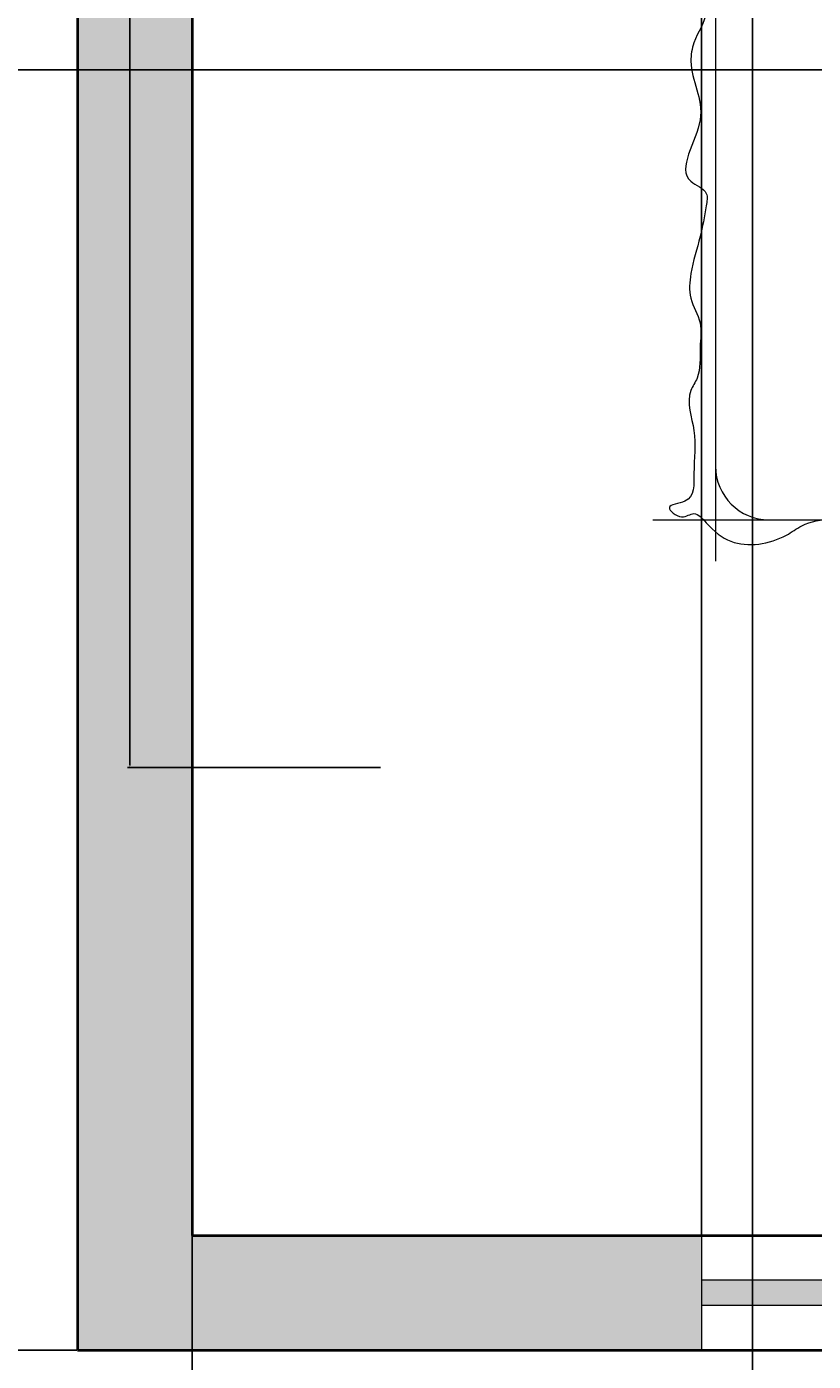
# Model space of a CAD drawing. Units: inches. Extents: x 2330 to 3943, y 1763 to 3461.
# Tile 3 of 40: x 2472 to 2533, y 2211 to 2316. Entities that reach past the tile are written whole.
import ezdxf

# ---------------------------------------------------------------- set-up
doc = ezdxf.new("R2010")
doc.units = ezdxf.units.IN
for name, color, linetype, lineweight in [('A-ANNO-DIMS', 2, 'Continuous', 18), ('A-FURN', 8, 'Continuous', 13), ('A-GLAZ', 4, 'Continuous', 18), ('A-WALL', 7, 'Continuous', 40), ('A-WALL-PATT', 252, 'Continuous', 13)]:
    doc.layers.add(name, color=color, linetype=linetype, lineweight=lineweight)
doc.styles.get("Standard").update_dxf_attribs({"font": 'arial.ttf'})
doc.dimstyles.get("Standard").update_dxf_attribs({"dimtxt": 0.18, "dimasz": 0.18, "dimexe": 0.18, "dimexo": 0.0625, "dimgap": 0.09, "dimtad": 0, "dimtih": 1, "dimtoh": 1, "dimdec": 4, "dimzin": 0, "dimdsep": 46, "dimtxsty": 'Standard', "dimcen": 0.09, "dimadec": 0, "dimazin": 0, "dimtfac": 1, "dimtdec": 4, "dimtofl": 0, "dimtmove": 0, "dimatfit": 3, "dimfxl": 1, "dimtolj": 1, "dimtzin": 0, "dimarcsym": 0})

# ---------------------------------------------------------------- blocks, each defined once
blk = doc.blocks.new('A$C200C7901')
for p, q in [((0.5, 1.3845), (0.5, 0.3086)), ((0.4061, 0.3703), (2.0386, 0.3703))]:
    blk.add_line(p, q)
blk.add_arc((0.58, 0.4503), 0.08, 180, 270)
blk.add_open_spline([(0.4856, 1.3429), (0.5504, 1.3182), (0.6715, 1.2721), (0.8374, 1.0498), (1.1164, 1.1183), (1.3878, 1.1816), (1.5888, 1.1102), (1.8403, 1.1127), (1.9415, 1.2178), (2.0032, 1.2819)], degree=3, knots=[0, 0, 0, 0, 205.411753, 383.654933, 772.067458, 921.644661, 1226.793228, 1388.983508, 1642.292305, 1642.292305, 1642.292305, 1642.292305])
at = {"linetype": 'ByBlock'}
blk.add_open_spline([(0.473, 1.2954), (0.4739, 1.2781), (0.4755, 1.2477), (0.5032, 1.2084), (0.4801, 1.1701), (0.4928, 1.1255), (0.4674, 1.0912), (0.4579, 1.0351), (0.501, 0.9724), (0.4311, 0.8832), (0.4902, 0.8637), (0.4843, 0.8288), (0.4774, 0.7906), (0.4625, 0.7457), (0.459, 0.6999), (0.4816, 0.6664), (0.4748, 0.625), (0.4791, 0.5889), (0.4533, 0.5528), (0.4738, 0.5004), (0.4658, 0.4502), (0.4696, 0.3946), (0.4189, 0.3935), (0.4493, 0.3684), (0.4694, 0.3857), (0.4922, 0.3576), (0.5297, 0.3262), (0.5917, 0.3353), (0.6454, 0.3754), (0.7083, 0.3741), (0.7643, 0.3328), (0.826, 0.346), (0.925, 0.3388), (1.0353, 0.3593), (1.1561, 0.3744), (1.2477, 0.3154), (1.3302, 0.3474), (1.4086, 0.3512), (1.5217, 0.3878), (1.6362, 0.3176), (1.7682, 0.3285), (1.8402, 0.3019), (1.9071, 0.3529), (1.9647, 0.3412), (2.0795, 0.2948), (2.0472, 0.3498), (2.0343, 0.3772), (2.0435, 0.43), (2.0109, 0.5782), (2.0746, 0.4643), (2.0805, 0.584), (2.0084, 0.5979), (2.0343, 0.6846), (2.0344, 0.746), (2.0293, 0.8096), (2.0489, 0.8545), (2.0652, 0.9218), (1.9842, 0.9297), (2.0007, 1.0162), (2.0367, 1.0585), (2.0367, 1.1102), (2.0457, 1.1647), (2.0226, 1.2084), (2.0234, 1.2306), (2.0236, 1.2352)], degree=3, knots=[0, 0, 0, 0, 51.660678, 90.967412, 128.902454, 170.303599, 219.852997, 247.834962, 336.321557, 429.35469, 458.821847, 477.222321, 524.135809, 581.038434, 617.839381, 657.146115, 693.947125, 740.178081, 760.753248, 820.731705, 885.133458, 928.777044, 953.563729, 976.574207, 995.553042, 1018.563482, 1064.584401, 1147.951297, 1174.787598, 1266.851571, 1308.018447, 1377.066427, 1441.511314, 1608.245014, 1714.11869, 1792.771707, 1913.247991, 1954.931389, 2029.864445, 2259.189419, 2305.221512, 2429.507982, 2456.344283, 2543.92595, 2627.925037, 2662.96218, 2687.736879, 2719.937755, 2839.540991, 2875.47895, 2953.681041, 2993.270313, 3066.872333, 3154.395764, 3200.397042, 3248.426375, 3312.828127, 3347.881398, 3444.484026, 3481.577522, 3518.665244, 3592.267265, 3644.719162, 3658.519501, 3658.519501, 3658.519501, 3658.519501], dxfattribs=at)
blk = doc.blocks.new('WINDOW-120IN')
h = blk.add_hatch(color=256)
h.dxf.hatch_style = 1
h.paths.add_polyline_path([(120, 5.5), (0, 5.5), (0, 3.5), (120, 3.5)])
for p, q in [((0, 9), (0, 0)), ((120, 9), (120, 0)), ((120, 5.5), (0, 5.5)), ((120, 3.5), (0, 3.5))]:
    blk.add_line(p, q)
blk = doc.blocks.new('*D40')
at = {"layer": 'A-ANNO-DIMS', "color": 0, "lineweight": -2, "transparency": 16777216}
for p, q in [((2499.44, 2380.43), (2479.59, 2380.43)), ((2479.77, 2380.25), (2479.77, 2319.34)), ((2479.77, 2258.07), (2479.77, 2318.98)), ((2499.44, 2257.89), (2479.59, 2257.89))]:
    blk.add_line(p, q, dxfattribs=at)
at = {"layer": 'A-ANNO-DIMS', "color": 0, "transparency": 16777216}
for points in [[(2479.74, 2380.25), (2479.8, 2380.25), (2479.77, 2380.43)], [(2479.74, 2258.07), (2479.8, 2258.07), (2479.77, 2257.89)]]:
    blk.add_solid(points, dxfattribs=at)
at = {"layer": 'Defpoints', "color": 0, "transparency": 16777216}
for p in [(2479.77, 2380.43), (2499.5, 2380.43), (2499.5, 2257.89)]:
    blk.add_point(p, dxfattribs=at)
at = {"layer": 'A-ANNO-DIMS', "color": 0, "transparency": 16777216, "insert": (2479.77, 2319.16), "char_height": 0.18, "attachment_point": 5}
blk.add_mtext('\\A1;123 TYP.', dxfattribs=at)
blk = doc.blocks.new('*D62')
at = {"layer": 'A-ANNO-DIMS', "color": 0, "lineweight": -2, "transparency": 16777216}
for p, q in [((2475.6, 3162.65), (2330.5, 3162.65)), ((2330.68, 3162.47), (2330.68, 2687.58)), ((2330.68, 2212.33), (2330.68, 2687.22)), ((2475.6, 2212.15), (2330.5, 2212.15))]:
    blk.add_line(p, q, dxfattribs=at)
at = {"layer": 'A-ANNO-DIMS', "color": 0, "transparency": 16777216}
for points in [[(2330.65, 3162.47), (2330.71, 3162.47), (2330.68, 3162.65)], [(2330.65, 2212.33), (2330.71, 2212.33), (2330.68, 2212.15)]]:
    blk.add_solid(points, dxfattribs=at)
at = {"layer": 'Defpoints', "color": 0, "transparency": 16777216}
for p in [(2330.68, 3162.65), (2475.66, 3162.65), (2475.66, 2212.15)]:
    blk.add_point(p, dxfattribs=at)
at = {"layer": 'A-ANNO-DIMS', "color": 0, "transparency": 16777216, "insert": (2330.68, 2687.4), "char_height": 0.18, "attachment_point": 5}
blk.add_mtext('\\A1;950.5', dxfattribs=at)
blk = doc.blocks.new('*D79')
at = {"layer": 'A-ANNO-DIMS', "color": 0, "lineweight": -2, "transparency": 16777216}
for p, q in [((2484.66, 2221.21), (2484.66, 3461.3)), ((2484.84, 3461.12), (2504.44, 3461.12)), ((2524.48, 3461.12), (2504.88, 3461.12)), ((2524.66, 2221.21), (2524.66, 3461.3))]:
    blk.add_line(p, q, dxfattribs=at)
at = {"layer": 'A-ANNO-DIMS', "color": 0, "transparency": 16777216}
for points in [[(2484.84, 3461.15), (2484.84, 3461.09), (2484.66, 3461.12)], [(2524.48, 3461.15), (2524.48, 3461.09), (2524.66, 3461.12)]]:
    blk.add_solid(points, dxfattribs=at)
at = {"layer": 'Defpoints', "color": 0, "transparency": 16777216}
for p in [(2524.66, 3461.12), (2484.66, 2221.15), (2524.66, 2221.15)]:
    blk.add_point(p, dxfattribs=at)
at = {"layer": 'A-ANNO-DIMS', "color": 0, "transparency": 16777216, "insert": (2504.66, 3461.12), "char_height": 0.18, "attachment_point": 5}
blk.add_mtext('\\A1;40', dxfattribs=at)
blk = doc.blocks.new('*D80')
at = {"layer": 'A-ANNO-DIMS', "color": 0, "lineweight": -2, "transparency": 16777216}
for p, q in [((3166.6, 2331.7), (2330.5, 2331.7)), ((2330.68, 2331.52), (2330.68, 2322.36)), ((2330.68, 2312.83), (2330.68, 2321.99)), ((3166.6, 2312.65), (2330.5, 2312.65))]:
    blk.add_line(p, q, dxfattribs=at)
at = {"layer": 'A-ANNO-DIMS', "color": 0, "transparency": 16777216}
for points in [[(2330.65, 2331.52), (2330.71, 2331.52), (2330.68, 2331.7)], [(2330.65, 2312.83), (2330.71, 2312.83), (2330.68, 2312.65)]]:
    blk.add_solid(points, dxfattribs=at)
at = {"layer": 'Defpoints', "color": 0, "transparency": 16777216}
for p in [(2330.68, 2331.7), (3166.66, 2331.7), (3166.66, 2312.65)]:
    blk.add_point(p, dxfattribs=at)
at = {"layer": 'A-ANNO-DIMS', "color": 0, "transparency": 16777216, "insert": (2330.68, 2322.18), "char_height": 0.18, "attachment_point": 5}
blk.add_mtext('\\A1;19.046', dxfattribs=at)
blk = doc.blocks.new('*D90')
at = {"layer": 'A-ANNO-DIMS', "color": 0, "lineweight": -2, "transparency": 16777216}
for p, q in [((2484.66, 3153.59), (2484.66, 1901.2)), ((2528.66, 3153.59), (2528.66, 1901.2)), ((2484.84, 1901.38), (2506.44, 1901.38)), ((2528.48, 1901.38), (2506.88, 1901.38))]:
    blk.add_line(p, q, dxfattribs=at)
at = {"layer": 'A-ANNO-DIMS', "color": 0, "transparency": 16777216}
for points in [[(2484.84, 1901.41), (2484.84, 1901.35), (2484.66, 1901.38)], [(2528.48, 1901.41), (2528.48, 1901.35), (2528.66, 1901.38)]]:
    blk.add_solid(points, dxfattribs=at)
at = {"layer": 'Defpoints', "color": 0, "transparency": 16777216}
for p in [(2484.66, 3153.65), (2528.66, 3153.65), (2528.66, 1901.38)]:
    blk.add_point(p, dxfattribs=at)
at = {"layer": 'A-ANNO-DIMS', "color": 0, "transparency": 16777216, "insert": (2506.66, 1901.38), "char_height": 0.18, "attachment_point": 5}
blk.add_mtext('\\A1;44', dxfattribs=at)

msp = doc.modelspace()

# ---------------------------------------------------------------- hatches: boundary and pattern name
at = {"layer": 'A-WALL-PATT'}
h = msp.add_hatch(color=256, dxfattribs=at)
h.dxf.hatch_style = 1
h.paths.add_polyline_path([(2484.6605, 2499.7574), (2475.6605, 2499.7574), (2475.6605, 2212.1524), (2524.6605, 2212.1524), (2524.6605, 2221.1524), (2484.6605, 2221.1524), (2484.6605, 2385.1524), (2624.6605, 2385.1524), (2624.6605, 2422.1524), (2619.6605, 2422.1524), (2619.6605, 2390.1524), (2484.6605, 2390.1524), (2484.6605, 2462.1524), (2553.7039, 2462.1524), (2553.7039, 2467.1524), (2484.6605, 2467.1524)])

# ---------------------------------------------------------------- linework, layer by layer
at = {"layer": 'A-WALL'}
for p, q in [((2475.6605, 3162.6524), (2475.6605, 2212.1524)), ((2484.6605, 2385.1524), (2484.6605, 2221.1524)), ((2484.6605, 2221.1524), (2684.6605, 2221.1524)), ((2475.6605, 2212.1524), (2693.6605, 2212.1524))]:
    msp.add_line(p, q, dxfattribs=at)

# ---------------------------------------------------------------- block references
at = {"layer": 'A-FURN', "xscale": 52.5181391560459, "yscale": 52.5181391560459, "zscale": 52.5181391560459}
msp.add_blockref('A$C200C7901', (2499.4987, 2257.8888), dxfattribs=at)
at = {"layer": 'A-GLAZ'}
msp.add_blockref('WINDOW-120IN', (2524.6605, 2212.1524), dxfattribs=at)

# ---------------------------------------------------------------- dimensions: what is measured, and where the dimension line sits
at = {"layer": 'A-ANNO-DIMS'}
for base, p1, p2, picture, middle in [((2524.6605, 3461.1231), (2484.6605, 2221.1524), (2524.6605, 2221.1524), '*D79', (2504.6605, 3461.1231)), ((2528.6605, 1901.3774), (2484.6605, 3153.6524), (2528.6605, 3153.6524), '*D90', (2506.6605, 1901.3774))]:
    dim = msp.add_linear_dim(base=base, p1=p1, p2=p2, dimstyle='Standard', override={"dimdec": 0, "dimlfac": 1, "dimrnd": 0, "dimzin": 0, "dimdsep": 46, "dimlunit": 2}, dxfattribs=at)
    dim.commit()
    dim.dimension.update_dxf_attribs({"geometry": picture, "text_midpoint": middle})
for base, p1, p2, override, picture, middle in [((2330.6824, 3162.6524), (2475.6605, 2212.1524), (2475.6605, 3162.6524), {"dimdec": 1, "dimlfac": 1, "dimrnd": 0, "dimzin": 0, "dimdsep": 46, "dimlunit": 2}, '*D62', (2330.6824, 2687.4024)), ((2330.6824, 2331.6982), (3166.6605, 2312.6524), (3166.6605, 2331.6982), {"dimdec": 3, "dimlfac": 1, "dimrnd": 0, "dimzin": 0, "dimdsep": 46, "dimlunit": 2}, '*D80', (2330.6824, 2322.1753))]:
    dim = msp.add_linear_dim(base=base, p1=p1, p2=p2, angle=90, dimstyle='Standard', override=override, dxfattribs=at)
    dim.commit()
    dim.dimension.update_dxf_attribs({"geometry": picture, "text_midpoint": middle})
dim = msp.add_linear_dim(base=(2479.7696, 2380.4339), p1=(2499.4986, 2257.8888), p2=(2499.4986, 2380.4339), angle=90, text='<> TYP.', dimstyle='Standard', override={"dimdec": 0, "dimlfac": 1, "dimrnd": 0, "dimzin": 0, "dimdsep": 46, "dimlunit": 2}, dxfattribs=at)
dim.commit()
dim.dimension.update_dxf_attribs({"geometry": '*D40', "text_midpoint": (2479.7696, 2319.1613)})

doc.saveas('drawing.dxf')
